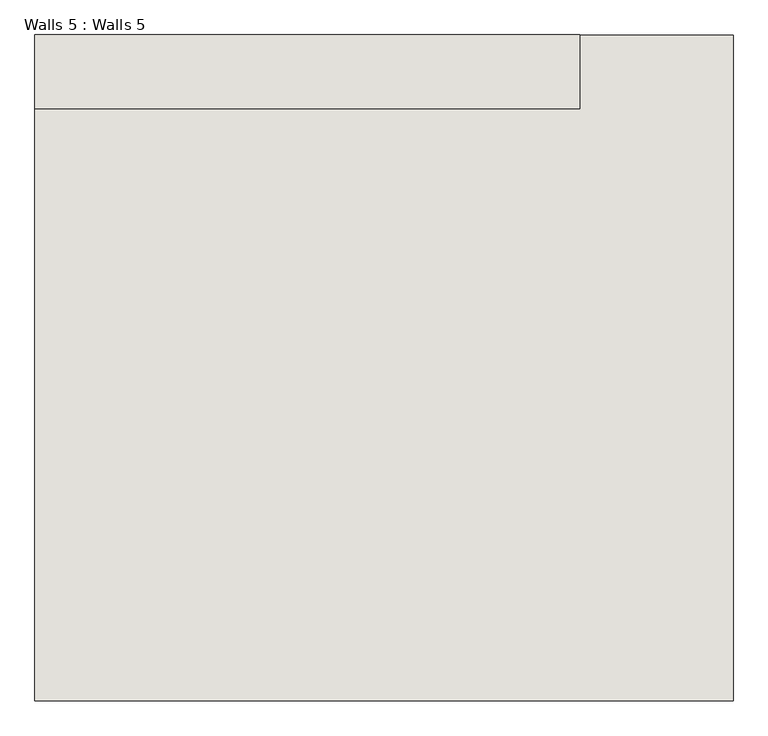
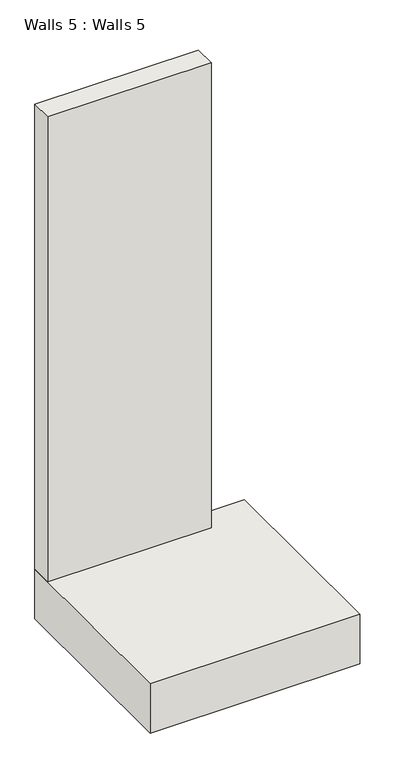
"""IFC4 building model written with IfcOpenShell, lengths in millimetres: wall geometry, Walls 5 : Walls 5."""

from ifc_helpers import new_model, si_unit, frame, origin, place, context, project, spatial, polyline, outline, extrude, source, transform, mapped, element, save


def walls_5_walls_5_4d7304d2(model_context):
    return source(origin(), model_context, "Body", "SweptSolid", [
        extrude(outline(polyline([(-11513.4620963, 3039.5114178), (-9227.4620963, 3039.5114178), (-9227.4620963, 2730.1130309), (-11513.4620963, 2730.1130309), (-11513.4620963, 3039.5114178)])), frame((0.0, 0.0, 4095.8208602), z_axis=(0.0, 0.0, 1.0), x_axis=(1.0, 0.0, 0.0)), (0.0, 0.0, 1.0), 6876.9791398),
        extrude(outline(polyline([(-11513.4620963, 245.5114178), (-11513.4620963, 3039.5114178), (-8584.5102765, 3039.5114178), (-8584.5102765, 245.5114178), (-11513.4620963, 245.5114178)])), frame((0.0, 0.0, 3367.4133314), z_axis=(0.0, 0.0, 1.0), x_axis=(1.0, 0.0, 0.0)), (0.0, 0.0, 1.0), 728.4075287),
    ])


if __name__ == "__main__":
    model = new_model("IFC4")
    model_context = context("Model", 3, world=origin())
    ifc_project = project(units=[si_unit("LENGTHUNIT", "METRE", prefix="MILLI")], contexts=[model_context])
    site = spatial("IfcSite", under=ifc_project)
    building = spatial("IfcBuilding", under=site)
    placement = place(None, origin())
    walls_5_walls_5_shape = walls_5_walls_5_4d7304d2(model_context)
    element("IfcWall", 1, ObjectType="Walls 5 : Walls 5", at=placement, inside=building, context=model_context, shape_type="MappedRepresentation", body=[
        mapped(walls_5_walls_5_shape, transform((0.0, 0.0, 0.0), x_axis=(1.0, 0.0, 0.0), y_axis=(0.0, 1.0, 0.0), z_axis=(0.0, 0.0, 1.0))),
    ])
    save(model, "model.ifc")

# Revit data of these elements
# Element 1 (IfcWall, "Walls 5 : Walls 5")
#   Materials on its faces: "Default Wall"
# Materials
#   "Default Wall": colour RGB 128 128 128, transparency 0
